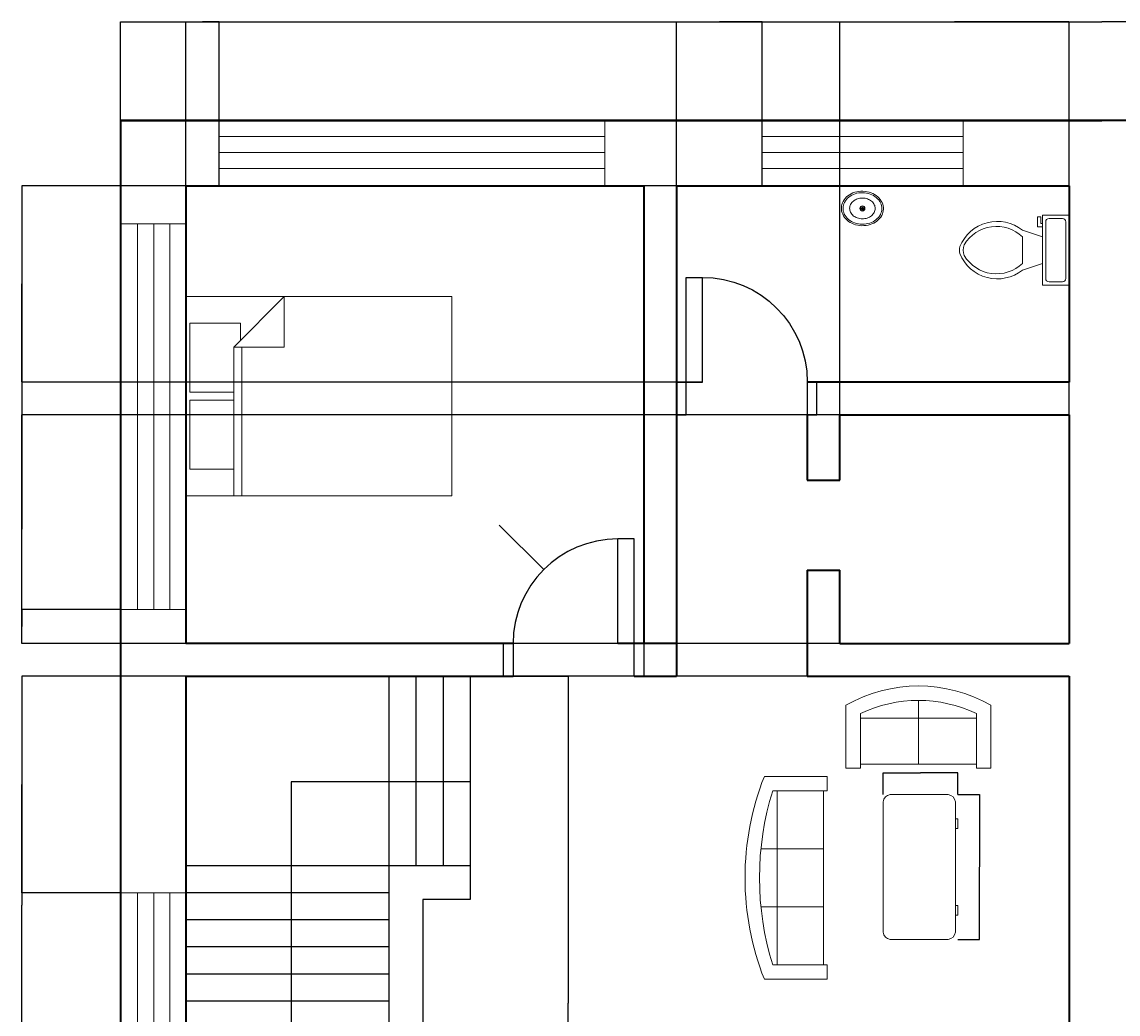
# Model space of a CAD drawing. Units: millimetres. Extents: x 726 to 37095, y -1634 to 13537.
# Tile 3 of 4: x 20550 to 28928, y 5952 to 13537. Entities that reach past the tile are written whole.
import ezdxf

# ---------------------------------------------------------------- set-up
doc = ezdxf.new("R2010")
doc.units = ezdxf.units.MM
for name, color, linetype, lineweight in [('A-ANNO-DIMS', 2, 'Continuous', 18), ('A-DOOR', 3, 'Continuous', 25), ('A-FLOR-FIXT', 9, 'Continuous', 18), ('A-FLOR-STRS', 5, 'Continuous', 25), ('A-FURN', 8, 'Continuous', 18), ('A-GLAZ', 4, 'Continuous', 18), ('A-WALL', 7, 'Continuous', 35)]:
    doc.layers.add(name, color=color, linetype=linetype, lineweight=lineweight)
doc.styles.get("Standard").update_dxf_attribs({"font": 'arial.ttf'})
doc.dimstyles.get("Standard").update_dxf_attribs({"dimtxt": 0.18, "dimasz": 0.18, "dimexe": 0.18, "dimexo": 0.0625, "dimgap": 0.09, "dimtad": 0, "dimtih": 1, "dimtoh": 1, "dimdec": 4, "dimzin": 0, "dimdsep": 46, "dimtxsty": 'Standard', "dimcen": 0.09, "dimadec": 0, "dimazin": 0, "dimtfac": 1, "dimtdec": 4, "dimtofl": 0, "dimtmove": 0, "dimatfit": 3, "dimfxl": 1, "dimtolj": 1, "dimtzin": 0, "dimarcsym": 0})

# ---------------------------------------------------------------- blocks, each defined once
blk = doc.blocks.new('Bed - Queen')
for p, q in [((0, -80.00003000000002), (0, 0)), ((0, 0), (59.99998999999999, 0)), ((59.99998999999999, 0), (59.99998999999999, -80.00003000000002)), ((7.99999, -1.200000000000017), (28.79998, -1.200000000000017)), ((7.99999, -14.4), (7.99999, -1.200000000000017)), ((28.79998, -1.200000000000017), (28.79998, -14.4)), ((31.19999, -1.200000000000017), (51.99999000000001, -1.200000000000017)), ((31.19999, -14.4), (31.19999, -1.200000000000017)), ((51.99999000000001, -1.200000000000017), (51.99999000000001, -16.4)), ((0, -14.4), (44.79999999999999, -14.4)), ((59.99998999999999, -29.60000000000001), (44.79999999999999, -14.4)), ((44.79999999999999, -14.4), (44.79999999999999, -29.60000000000001)), ((51.99999000000001, -16.4), (46.79936, -16.4)), ((44.79999999999999, -16.80000000000001), (0, -16.80000000000001)), ((44.79999999999999, -29.60000000000001), (59.99998999999999, -29.60000000000001)), ((59.99998999999999, -80.00003000000002), (0, -80.00003000000002))]:
    blk.add_line(p, q)
blk = doc.blocks.new('Window - Wood Frame 36 in. Wide plan')
for p, q in [((0, 6), (0, 0)), ((36, 6), (36, 0)), ((0, 4.5), (36, 4.5)), ((0, 3), (36, 3)), ((0, 1.5), (36, 1.5))]:
    blk.add_line(p, q)
blk = doc.blocks.new('Sofa - Roundback 7 ft.')
for p, q in [((-12.00002, -32.44210000000393), (-12.00003, -6.597100000003898)), ((11.99996999999999, -32.44210000000393), (11.99997999999999, -6.597100000003898)), ((-36.000027, -34.00000000000395), (-36.000027, -11.46960000000396)), ((-35.999844, -13.38190000000397), (35.99979999999999, -13.38190000000397)), ((35.99997999999999, -34.00000000000395), (35.99997999999999, -11.46960000000396)), ((-36.000027, -32.44210000000393), (35.99997999999999, -32.44210000000393))]:
    blk.add_line(p, q)
for points in [[(-36.000027, -34.00000000000395), (-42.000027, -34.00000000000395), (-42.000027, -8.000000000003944)], [(41.99997999999999, -8.000000000003944), (41.99997999999999, -34.00000000000395), (35.99997999999999, -34.00000000000395)]]:
    blk.add_lwpolyline(points)
for centre, radius, start, end in [((0, -114.2500000000039), 114.2500000000039, 68.43141000000072, 111.5686000000006), ((-1.00000000032e-05, -127.1968000000039), 121.1967999999973, 72.72032999999948, 107.2797000000005)]:
    blk.add_arc(centre, radius, start, end)
blk = doc.blocks.new('Desk - 30 x 60 in.')
for p, q in [((-26.999995, 0), (26.999995, 0)), ((-29.999995, -27), (-29.999995, -3)), ((29.999995, -3), (29.999995, -27)), ((26.999995, -30), (-26.999995, -30)), ((-20.000005, -30), (-20.000005, -31)), ((-20.000005, -31), (-16.000005, -31)), ((-16.000005, -31), (-16.000005, -30)), ((15.999995, -31), (15.999995, -30)), ((19.999995, -31), (15.999995, -31)), ((19.999995, -30), (19.999995, -31))]:
    blk.add_line(p, q)
for centre, radius, start, end in [((-26.499995, -3.5), 3.535534000004229, 98.1300999999916, 171.8698999999352), ((26.499995, -3.5), 3.535533999997753, 8.130102000022115, 81.8698999999439), ((-26.499995, -26.5), 3.535534000000845, 188.1301000000653, 261.8699000000085), ((26.499995, -26.5), 3.535534000004826, 278.1301000000561, 351.8698999999439)]:
    blk.add_arc(centre, radius, start, end)
blk = doc.blocks.new('Sofa - Roundback Loveseat 5 ft.')
for p, q in [((0, -32.44198000000246), (0, -5.999980000002448)), ((-23.99999999999999, -33.99998000000245), (-23.99999999999999, -11.46958000000243)), ((-23.99979999999998, -13.38178000000245), (23.99986, -13.38178000000245)), ((24.00004000000001, -33.99998000000245), (24.00004000000001, -11.46958000000243)), ((-23.99999999999999, -32.44198000000246), (24.00004000000001, -32.44198000000246))]:
    blk.add_line(p, q)
for points in [[(-23.99999999999999, -33.99998000000245), (-29.99999999999999, -33.99998000000245), (-29.99999999999999, -7.999980000002448)], [(30.00004000000001, -7.999980000002448), (30.00004000000001, -33.99998000000245), (24.00004000000001, -33.99998000000245)]]:
    blk.add_lwpolyline(points)
for centre, radius, start, end in [((0, -60.24998000000245), 60.24998000000245, 60.13715000000122, 119.862800000004), ((0, -61.38438000000245), 55.38444000000723, 64.32083000000306, 115.6791999999996)]:
    blk.add_arc(centre, radius, start, end)
blk = doc.blocks.new('Toilet - top')
for p, q in [((9.5, -6), (9.5, -2)), ((-10, -8.5), (-8, -8.5)), ((-10, -9.5), (-10, -8.5)), ((-7, -9.5), (-10, -9.5)), ((-8, -8.5), (-8, -8)), ((-7, -8), (-7, -9.5)), ((-4, -8), (-6, -14)), ((4, -8), (6, -14)), ((4, -14), (-4, -14))]:
    blk.add_line(p, q)
blk.add_lwpolyline([(10.5, -8), (10.5, 0), (-10.5, 0), (-10.5, -8)], close=True)
for points in [[(-9.5, -2), (-9.5, -6)], [(8.5, -1), (-8.5, -1)], [(-8.5, -7), (8.5, -7)]]:
    blk.add_lwpolyline(points)
for centre, radius, start, end in [((-8.625, -1.875), 0.8838834999999999, 81.86989999999999, 188.1301), ((8.625, -1.875), 0.8838834999999999, 351.8699, 98.13009999999998), ((-8.625, -6.125), 0.8838834999999999, 171.869898, 278.1301), ((8.625, -6.125), 0.8838834999999999, 261.8699, 8.130099999999993), ((3.519562435188956, -21.58049502388982), 12.16902005083646, 141.4691096810948, 247.9714346835576), ((4.199957580658807, -21.81740929088453), 11.3291791325804, 136.3677254423718, 238.946823937405), ((-3.519499936778316, -21.58047137067522), 12.16903423757823, 292.0284332733152, 38.53070636800453), ((-4.199890672038477, -21.81738596564128), 11.32918622148567, 301.0530065773863, 43.63209216694732), ((2.09660981727e-05, -27.87646475467881), 4, 245.7318247449371, 294.2681740488959), ((2.09415214183e-05, -28.99996806116075), 4, 254.8605283244437, 285.1394707718433)]:
    blk.add_arc(centre, radius, start, end)
blk = doc.blocks.new('Sink - Oval top')
for p, q in [((-1, 0), (1, 0)), ((0, 1), (0, -1))]:
    blk.add_line(p, q)
for points in [[(-12.23371880354079, 0.3941914712607968, 0.1176342565883263), (-11.46456229543957, -3.361933235489118, 0.104469279667093), (-8.878748691070427, -6.803541973650567, 0.0900157896014849), (-5.082757700676665, -9.072309807490512, 0.0819199491592185), (-0.3227280122732736, -10.01585280257211, 0.0819199491592091), (4.488169920880977, -9.380701564817912, 0.0900157896014801), (8.422342359155778, -7.36101289847943, 0.1044692796670922), (11.22435122606941, -4.093009071543406, 0.1176342565883338), (12.23371880354091, -0.3941914712607968, 0.1176342565883057), (11.46456229543992, 3.361933235488777, 0.1044692796670849), (8.878748691070427, 6.803541973650567, 0.0900157896014884), (5.082757700676324, 9.072309807490681, 0.0819199491592058), (0.3227280122732736, 10.01585280257211, 0.081919949159207), (-4.488169920880864, 9.380701564817969, 0.0900157896014802), (-8.422342359155778, 7.36101289847943, 0.1044692796670951), (-11.22435122606919, 4.093009071543633, 0.1176342565883402)], [(-11.28627986850119, 0.1590597164737346, 0.1186217001864142), (-10.51590095791209, -3.253161772358112, 0.1046781721811095), (-8.071803350560115, -6.358618019863342, 0.0895620664691738), (-4.537699193222351, -8.366971929609804, 0.0811846988912177), (-0.1289739026695997, -9.15150355811437, 0.0811846988912276), (4.300109150126218, -8.491524865184601, 0.0895620664691798), (7.889406708212618, -6.583562428127606, 0.1046781721811044), (10.42004782883111, -3.548216131892445, 0.1186217001864013), (11.28627986850119, -0.1590597164736209, 0.1186217001863945), (10.51590095791221, 3.253161772357998, 0.1046781721811069), (8.071803350560115, 6.358618019863342, 0.0895620664691756), (4.537699193222124, 8.366971929609917, 0.081184698891216), (0.1289739026695997, 9.151503558114428, 0.0811846988912142), (-4.300109150125877, 8.491524865184829, 0.0895620664691747), (-7.889406708212618, 6.583562428127606, 0.1046781721811045), (-10.42004782883111, 3.548216131892445, 0.1186217001863946)], [(-7.420452389032902, 0.0829876781601797, 0.1182825673856775), (-6.907065465214486, -2.1674649380775, 0.1046074595377274), (-5.294791470712084, -4.209988192029413, 0.0897179636260996), (-2.966599981142508, -5.528122152688069, 0.0814360825277113), (-0.0675135187855176, -6.036810076758797, 0.0814360825277218), (2.84222437824053, -5.593085960977873, 0.0897179636261315), (5.199312936802016, -4.327350491993342, 0.1046074595376878), (6.85686365682659, -2.321395784920355, 0.1182825673856714), (7.420452389033016, -0.0829876781601797, 0.1182825673856961), (6.907065465214486, 2.167464938077614, 0.1046074595377135), (5.294791470712084, 4.209988192029413, 0.0897179636261265), (2.966599981142621, 5.528122152687842, 0.0814360825277426), (0.0675135187855176, 6.036810076758797, 0.0814360825277225), (-2.842224378240644, 5.593085960977873, 0.0897179636261212), (-5.199312936802016, 4.327350491993342, 0.1046074595377049), (-6.856863656826476, 2.321395784920355, 0.1182825673856712)]]:
    blk.add_lwpolyline(points, format="xyb", close=True)
for radius in [1.5, 1]:
    blk.add_circle((0, 0), radius)
blk = doc.blocks.new('DOOR-SWING-800')
for p, q in [((999.1999999999979, 1050), (874.1999999999979, 1050)), ((874.1999999999979, 250), (874.1999999999979, 1050)), ((999.1999999999979, 250), (999.1999999999979, 1050)), ((9.095e-13, 250), (74.199999999998, 250)), ((9.095e-13, 0), (9.095e-13, 250)), ((74.199999999998, 250), (74.199999999998, 0)), ((874.1999999999979, 250), (999.1999999999979, 250)), ((999.1999999999979, 250), (1073.400000000002, 250)), ((999.1999999999979, 0), (999.1999999999979, 250)), ((1073.400000000002, 250), (1073.400000000002, 0)), ((74.199999999998, 0), (9.095e-13, 0)), ((1073.400000000002, 0), (999.1999999999979, 0))]:
    blk.add_line(p, q)
blk.add_arc((874.1999999999979, 250), 800, 90, 180)
blk = doc.blocks.new('STAIR-QUARTER-TURN')
for p, q in [((1551.94660387568, 5000.000000000002), (1551.94660387568, 3551.516503049365)), ((1758.872817725773, 5000.000000000002), (1758.872817725773, 3551.516503049365)), ((1965.799031575862, 5000.000000000002), (1965.799031575862, 3551.516503049365)), ((2172.725245425954, 5000.000000000002), (2172.725245425954, 3551.516503049365)), ((2172.725245425954, 4193.579423830473), (803.743340616409, 4193.579423830471)), ((803.743340616409, 4193.579423830471), (803.743340616409, 330.5564002077117)), ((2172.725245425954, 3551.516503049366), (0, 3551.516503049365)), ((1551.94660387568, 3551.516503049365), (1551.94660387568, 3344.590289199272)), ((2172.725245425954, 3551.516503049365), (2172.725245425954, 3292.858735736751)), ((1551.94660387568, 3344.590289199272), (0, 3344.590289199273)), ((1551.94660387568, 3344.590289199272), (1551.94660387568, 861.4757229981805)), ((2172.725245425954, 3292.858735736751), (1810.604371188295, 3292.858735736751)), ((1810.604371188295, 3292.85873573675), (1810.604371188295, 602.8179556856148)), ((1551.94660387568, 3137.664075349182), (0, 3137.664075349182)), ((1551.94660387568, 2930.73786149909), (0, 2930.737861499091)), ((1551.94660387568, 2723.811647649), (0, 2723.811647649001)), ((1551.94660387568, 2516.885433798908), (0, 2516.885433798909)), ((1551.94660387568, 2309.959219948817), (0, 2309.959219948818)), ((1551.94660387568, 2103.033006098726), (0, 2103.033006098727)), ((1551.94660387568, 1896.106792248635), (0, 1896.106792248635)), ((1551.94660387568, 1689.180578398543), (0, 1689.180578398544)), ((1551.94660387568, 1482.254364548453), (0, 1482.254364548454)), ((1551.94660387568, 1275.328150698362), (0, 1275.328150698363)), ((1551.94660387568, 1068.40193684827), (0, 1068.401936848271)), ((1551.94660387568, 861.4757229981795), (0, 861.4757229981805)), ((1551.94660387568, 861.4757229981805), (1551.946603875687, 602.8179556856074)), ((1810.604371188295, 602.8179556856148), (1551.946603875687, 602.8179556855675)), ((803.743340616409, 330.5564002077117), (545.0855733037969, 330.5564002077117)), ((545.0855733037969, 330.5564002077117), (803.743340616409, 4.547e-13)), ((803.743340616409, 330.5564002077117), (1062.401107929021, 330.5564002077108)), ((803.743340616409, 4.547e-13), (1062.401107929021, 330.5564002077117))]:
    blk.add_line(p, q)
blk = doc.blocks.new('WIN-1535')
for p, q in [((0, 1.819e-12), (0, 500.0000000000036)), ((1534.861597237876, 1.819e-12), (1534.861597237876, 500.0000000000036)), ((-9.095e-13, 377.1532172399693), (1534.861597237876, 377.1532172399693)), ((-9.095e-13, 254.306434479935), (1534.861597237876, 254.306434479935)), ((-9.095e-13, 131.459651719897), (1534.861597237876, 131.4596517198988))]:
    blk.add_line(p, q)
blk = doc.blocks.new('*D29')
at = {"layer": 'A-ANNO-DIMS', "color": 0, "lineweight": -2, "transparency": 16777216}
for p, q in [((27704.03518192463, 7629.827471204357), (27870.29711232547, 7629.827471204357)), ((27870.11711232547, 7629.647471204356), (27870.11711232547, 7076.195772778692)), ((27870.11711232547, 6522.377935198867), (27870.11711232547, 7075.829633624531)), ((27704.03518192463, 6522.197935198867), (27870.29711232547, 6522.197935198867))]:
    blk.add_line(p, q, dxfattribs=at)
at = {"layer": 'A-ANNO-DIMS', "color": 0, "transparency": 16777216}
for points in [[(27870.08711232547, 7629.647471204356), (27870.14711232546, 7629.647471204356), (27870.11711232547, 7629.827471204357)], [(27870.08711232547, 6522.377935198867), (27870.14711232546, 6522.377935198867), (27870.11711232547, 6522.197935198867)]]:
    blk.add_solid(points, dxfattribs=at)
at = {"layer": 'Defpoints', "color": 0, "transparency": 16777216}
for p in [(27703.97268192463, 7629.827471204357), (27870.11711232547, 7629.827471204357), (27703.97268192463, 6522.197935198867)]:
    blk.add_point(p, dxfattribs=at)
at = {"layer": 'A-ANNO-DIMS', "color": 0, "transparency": 16777216, "insert": (27870.11711232546, 7076.012703201602), "char_height": 0.18, "attachment_point": 5}
blk.add_mtext('\\A1;DESK 1108 TYP.', dxfattribs=at)
blk = doc.blocks.new('*D30')
at = {"layer": 'A-ANNO-DIMS', "color": 0, "lineweight": -2, "transparency": 16777216}
for p, q in [((27131.69732634582, 7629.889971204353), (27131.69732634582, 7796.151901605177)), ((27131.87732634582, 7795.971901605176), (27417.2369891284, 7795.971901605176)), ((27703.79268192461, 7795.971901605176), (27418.43301914204, 7795.971901605176)), ((27703.97268192462, 7629.889971204353), (27703.97268192462, 7796.151901605177))]:
    blk.add_line(p, q, dxfattribs=at)
at = {"layer": 'A-ANNO-DIMS', "color": 0, "transparency": 16777216}
for points in [[(27131.87732634582, 7796.001901605176), (27131.87732634582, 7795.941901605177), (27131.69732634582, 7795.971901605176)], [(27703.79268192461, 7796.001901605176), (27703.79268192461, 7795.941901605177), (27703.97268192462, 7795.971901605176)]]:
    blk.add_solid(points, dxfattribs=at)
at = {"layer": 'Defpoints', "color": 0, "transparency": 16777216}
for p in [(27131.69732634582, 7795.971901605176), (27131.69732634582, 7629.827471204354), (27703.97268192462, 7629.827471204354)]:
    blk.add_point(p, dxfattribs=at)
at = {"layer": 'A-ANNO-DIMS', "color": 0, "transparency": 16777216, "insert": (27417.83500413522, 7795.971901605176), "char_height": 0.18, "attachment_point": 5}
blk.add_mtext('\\A1;572 TYP.', dxfattribs=at)
blk = doc.blocks.new('*D35')
at = {"layer": 'A-ANNO-DIMS', "color": 0, "lineweight": -2, "transparency": 16777216}
for p, q in [((23976.18779894455, 8533.885868122888), (24726.30529894457, 8533.885868122888)), ((24726.12529894457, 8533.705868122888), (24726.12529894457, 6034.068937699966)), ((24726.12529894457, 3534.065868122886), (24726.12529894457, 6033.702798545806)), ((23976.18779894455, 3533.885868122886), (24726.30529894458, 3533.885868122886))]:
    blk.add_line(p, q, dxfattribs=at)
at = {"layer": 'A-ANNO-DIMS', "color": 0, "transparency": 16777216}
for points in [[(24726.09529894457, 8533.705868122888), (24726.15529894457, 8533.705868122888), (24726.12529894457, 8533.885868122888)], [(24726.09529894458, 3534.065868122886), (24726.15529894457, 3534.065868122886), (24726.12529894457, 3533.885868122886)]]:
    blk.add_solid(points, dxfattribs=at)
at = {"layer": 'Defpoints', "color": 0, "transparency": 16777216}
for p in [(23976.12529894455, 8533.885868122888), (24726.12529894457, 8533.885868122888), (23976.12529894455, 3533.885868122886)]:
    blk.add_point(p, dxfattribs=at)
at = {"layer": 'A-ANNO-DIMS', "color": 0, "transparency": 16777216, "insert": (24726.12529894457, 6033.885868122878), "char_height": 0.18, "attachment_point": 5}
blk.add_mtext('\\A1;STAIR 5000 TYP.', dxfattribs=at)
blk = doc.blocks.new('*D63')
at = {"layer": 'A-ANNO-DIMS', "color": 0, "lineweight": -2, "transparency": 16777216}
for p, q in [((21303.400054, 12783.948368), (21303.400054, 13536.815868)), ((21303.580054, 13536.635868), (28802.98013585539, 13536.635868)), ((36303.220054, 13536.635868), (28803.81997214461, 13536.635868)), ((36303.400054, 12783.948368), (36303.400054, 13536.815868))]:
    blk.add_line(p, q, dxfattribs=at)
at = {"layer": 'A-ANNO-DIMS', "color": 0, "transparency": 16777216}
for points in [[(21303.580054, 13536.665868), (21303.580054, 13536.605868), (21303.400054, 13536.635868)], [(36303.220054, 13536.665868), (36303.220054, 13536.605868), (36303.400054, 13536.635868)]]:
    blk.add_solid(points, dxfattribs=at)
at = {"layer": 'Defpoints', "color": 0, "transparency": 16777216}
for p in [(36303.400054, 13536.635868), (21303.400054, 12783.885868), (36303.400054, 12783.885868)]:
    blk.add_point(p, dxfattribs=at)
at = {"layer": 'A-ANNO-DIMS', "color": 0, "transparency": 16777216, "insert": (28803.400054, 13536.635868), "char_height": 0.18, "attachment_point": 5}
blk.add_mtext('\\A1;15000', dxfattribs=at)
blk = doc.blocks.new('*D69')
at = {"layer": 'A-ANNO-DIMS', "color": 0, "lineweight": -2, "transparency": 16777216}
for p, q in [((25303.33755400002, 12283.885868), (20550.47005400002, 12283.885868)), ((20550.65005400002, 12283.705868), (20550.65005400002, 10534.06783252933)), ((20550.65005400002, 8784.065868000003), (20550.65005400002, 10533.70390347067)), ((25303.33755400002, 8783.885868000005), (20550.47005400002, 8783.885868000005))]:
    blk.add_line(p, q, dxfattribs=at)
at = {"layer": 'A-ANNO-DIMS', "color": 0, "transparency": 16777216}
for points in [[(20550.62005400002, 12283.705868), (20550.68005400002, 12283.705868), (20550.65005400002, 12283.885868)], [(20550.62005400002, 8784.065868000003), (20550.68005400002, 8784.065868000003), (20550.65005400002, 8783.885868000005)]]:
    blk.add_solid(points, dxfattribs=at)
at = {"layer": 'Defpoints', "color": 0, "transparency": 16777216}
for p in [(20550.65005400002, 12283.885868), (25303.40005400002, 12283.885868), (25303.40005400002, 8783.885868000005)]:
    blk.add_point(p, dxfattribs=at)
at = {"layer": 'A-ANNO-DIMS', "color": 0, "transparency": 16777216, "insert": (20550.65005400002, 10533.88586799999), "char_height": 0.18, "attachment_point": 5}
blk.add_mtext('\\A1;3500', dxfattribs=at)
blk = doc.blocks.new('*D70')
at = {"layer": 'A-ANNO-DIMS', "color": 0, "lineweight": -2, "transparency": 16777216}
for p, q in [((25553.33755400002, 12283.885868), (20550.47005400002, 12283.885868)), ((20550.65005400002, 12283.705868), (20550.65005400002, 11534.06777113779)), ((20550.65005400002, 10784.065868), (20550.65005400002, 11533.70396486221)), ((25553.33755400002, 10783.885868), (20550.47005400002, 10783.885868))]:
    blk.add_line(p, q, dxfattribs=at)
at = {"layer": 'A-ANNO-DIMS', "color": 0, "transparency": 16777216}
for points in [[(20550.62005400002, 12283.705868), (20550.68005400002, 12283.705868), (20550.65005400002, 12283.885868)], [(20550.62005400002, 10784.065868), (20550.68005400002, 10784.065868), (20550.65005400002, 10783.885868)]]:
    blk.add_solid(points, dxfattribs=at)
at = {"layer": 'Defpoints', "color": 0, "transparency": 16777216}
for p in [(25553.40005400002, 12283.885868), (20550.65005400002, 10783.885868), (25553.40005400002, 10783.885868)]:
    blk.add_point(p, dxfattribs=at)
at = {"layer": 'A-ANNO-DIMS', "color": 0, "transparency": 16777216, "insert": (20550.65005400002, 11533.88586799999), "char_height": 0.18, "attachment_point": 5}
blk.add_mtext('\\A1;1500', dxfattribs=at)
blk = doc.blocks.new('*D71')
at = {"layer": 'A-ANNO-DIMS', "color": 0, "lineweight": -2, "transparency": 16777216}
for p, q in [((26802.600054, 10533.948368), (26802.600054, 13536.815868)), ((26802.780054, 13536.635868), (27677.54471293588, 13536.635868)), ((28553.220054, 13536.635868), (27678.45539506412, 13536.635868)), ((28553.400054, 10533.948368), (28553.400054, 13536.815868))]:
    blk.add_line(p, q, dxfattribs=at)
at = {"layer": 'A-ANNO-DIMS', "color": 0, "transparency": 16777216}
for points in [[(26802.780054, 13536.665868), (26802.780054, 13536.605868), (26802.600054, 13536.635868)], [(28553.220054, 13536.665868), (28553.220054, 13536.605868), (28553.400054, 13536.635868)]]:
    blk.add_solid(points, dxfattribs=at)
at = {"layer": 'Defpoints', "color": 0, "transparency": 16777216}
for p in [(28553.400054, 13536.635868), (26802.600054, 10533.885868), (28553.400054, 10533.885868)]:
    blk.add_point(p, dxfattribs=at)
at = {"layer": 'A-ANNO-DIMS', "color": 0, "transparency": 16777216, "insert": (27678.000054, 13536.635868), "char_height": 0.18, "attachment_point": 5}
blk.add_mtext('\\A1;1750.8', dxfattribs=at)
blk = doc.blocks.new('*D72')
at = {"layer": 'A-ANNO-DIMS', "color": 0, "lineweight": -2, "transparency": 16777216}
for p, q in [((28553.33755400002, 10533.885868), (20550.47005400002, 10533.885868)), ((20550.65005400002, 10533.705868), (20550.65005400002, 9659.067771137792)), ((20550.65005400002, 8784.065868000003), (20550.65005400002, 9658.703964862214)), ((28553.33755400002, 8783.885868000005), (20550.47005400002, 8783.885868000005))]:
    blk.add_line(p, q, dxfattribs=at)
at = {"layer": 'A-ANNO-DIMS', "color": 0, "transparency": 16777216}
for points in [[(20550.62005400002, 10533.705868), (20550.68005400002, 10533.705868), (20550.65005400002, 10533.885868)], [(20550.62005400002, 8784.065868000003), (20550.68005400002, 8784.065868000003), (20550.65005400002, 8783.885868000005)]]:
    blk.add_solid(points, dxfattribs=at)
at = {"layer": 'Defpoints', "color": 0, "transparency": 16777216}
for p in [(28553.40005400002, 10533.885868), (20550.65005400002, 8783.885868000005), (28553.40005400002, 8783.885868000005)]:
    blk.add_point(p, dxfattribs=at)
at = {"layer": 'A-ANNO-DIMS', "color": 0, "transparency": 16777216, "insert": (20550.65005400002, 9658.885867999996), "char_height": 0.18, "attachment_point": 5}
blk.add_mtext('\\A1;1750', dxfattribs=at)
blk = doc.blocks.new('*D73')
at = {"layer": 'A-ANNO-DIMS', "color": 0, "lineweight": -2, "transparency": 16777216}
for p, q in [((28553.33755400002, 8533.885868000005), (20550.47005400001, 8533.885868000005)), ((20550.65005400001, 8533.705868000003), (20550.65005400002, 6784.067832529334)), ((20550.65005400002, 5034.065868000002), (20550.65005400002, 6783.70390347067)), ((28553.33755400002, 5033.885868000002), (20550.47005400002, 5033.885868000002))]:
    blk.add_line(p, q, dxfattribs=at)
at = {"layer": 'A-ANNO-DIMS', "color": 0, "transparency": 16777216}
for points in [[(20550.62005400001, 8533.705868000003), (20550.68005400001, 8533.705868000003), (20550.65005400001, 8533.885868000005)], [(20550.62005400002, 5034.065868000002), (20550.68005400002, 5034.065868000002), (20550.65005400002, 5033.885868000002)]]:
    blk.add_solid(points, dxfattribs=at)
at = {"layer": 'Defpoints', "color": 0, "transparency": 16777216}
for p in [(20550.65005400001, 8533.885868000005), (28553.40005400002, 8533.885868000005), (28553.40005400002, 5033.885868000002)]:
    blk.add_point(p, dxfattribs=at)
at = {"layer": 'A-ANNO-DIMS', "color": 0, "transparency": 16777216, "insert": (20550.65005400001, 6783.885867999995), "char_height": 0.18, "attachment_point": 5}
blk.add_mtext('\\A1;3500', dxfattribs=at)
blk = doc.blocks.new('*D75')
at = {"layer": 'A-ANNO-DIMS', "color": 0, "lineweight": -2, "transparency": 16777216}
for p, q in [((28553.400054, 12283.948368), (28553.400054, 13536.815868)), ((28553.580054, 13536.635868), (28803.11151375444, 13536.635868)), ((29053.220054, 13536.635868), (28803.68859424557, 13536.635868)), ((29053.400054, 12283.948368), (29053.400054, 13536.815868))]:
    blk.add_line(p, q, dxfattribs=at)
at = {"layer": 'A-ANNO-DIMS', "color": 0, "transparency": 16777216}
for points in [[(28553.580054, 13536.665868), (28553.580054, 13536.605868), (28553.400054, 13536.635868)], [(29053.220054, 13536.665868), (29053.220054, 13536.605868), (29053.400054, 13536.635868)]]:
    blk.add_solid(points, dxfattribs=at)
at = {"layer": 'Defpoints', "color": 0, "transparency": 16777216}
for p in [(29053.400054, 13536.635868), (28553.400054, 12283.885868), (29053.400054, 12283.885868)]:
    blk.add_point(p, dxfattribs=at)
at = {"layer": 'A-ANNO-DIMS', "color": 0, "transparency": 16777216, "insert": (28803.400054, 13536.635868), "char_height": 0.18, "attachment_point": 5}
blk.add_mtext('\\A1;500', dxfattribs=at)
blk = doc.blocks.new('*D76')
at = {"layer": 'A-ANNO-DIMS', "color": 0, "lineweight": -2, "transparency": 16777216}
for p, q in [((25553.400054, 12283.948368), (25553.400054, 13536.815868)), ((25553.580054, 13536.635868), (25880.4339327367, 13536.635868)), ((26208.07657, 13536.635868), (25881.2226912633, 13536.635868)), ((26208.25657, 12283.948368), (26208.25657, 13536.815868))]:
    blk.add_line(p, q, dxfattribs=at)
at = {"layer": 'A-ANNO-DIMS', "color": 0, "transparency": 16777216}
for points in [[(25553.580054, 13536.665868), (25553.580054, 13536.605868), (25553.400054, 13536.635868)], [(26208.07657, 13536.665868), (26208.07657, 13536.605868), (26208.25657, 13536.635868)]]:
    blk.add_solid(points, dxfattribs=at)
at = {"layer": 'Defpoints', "color": 0, "transparency": 16777216}
for p in [(26208.25657, 13536.635868), (25553.400054, 12283.885868), (26208.25657, 12283.885868)]:
    blk.add_point(p, dxfattribs=at)
at = {"layer": 'A-ANNO-DIMS', "color": 0, "transparency": 16777216, "insert": (25880.828312, 13536.635868), "char_height": 0.18, "attachment_point": 5}
blk.add_mtext('\\A1;654.9', dxfattribs=at)
blk = doc.blocks.new('*D78')
at = {"layer": 'A-ANNO-DIMS', "color": 0, "lineweight": -2, "transparency": 16777216}
for p, q in [((21803.400054, 12283.948368), (21803.400054, 13536.815868)), ((21803.580054, 13536.635868), (21930.19670510437, 13536.635868)), ((22057.603097, 13536.635868), (21930.98644589564, 13536.635868)), ((22057.783097, 12292.561237), (22057.783097, 13536.815868))]:
    blk.add_line(p, q, dxfattribs=at)
at = {"layer": 'A-ANNO-DIMS', "color": 0, "transparency": 16777216}
for points in [[(21803.580054, 13536.665868), (21803.580054, 13536.605868), (21803.400054, 13536.635868)], [(22057.603097, 13536.665868), (22057.603097, 13536.605868), (22057.783097, 13536.635868)]]:
    blk.add_solid(points, dxfattribs=at)
at = {"layer": 'Defpoints', "color": 0, "transparency": 16777216}
for p in [(22057.783097, 13536.635868), (21803.400054, 12283.885868), (22057.783097, 12292.498737)]:
    blk.add_point(p, dxfattribs=at)
at = {"layer": 'A-ANNO-DIMS', "color": 0, "transparency": 16777216, "insert": (21930.5915755, 13536.635868), "char_height": 0.18, "attachment_point": 5}
blk.add_mtext('\\A1;254.4', dxfattribs=at)
blk = doc.blocks.new('*D80')
at = {"layer": 'A-ANNO-DIMS', "color": 0, "lineweight": -2, "transparency": 16777216}
for p, q in [((21803.33755400001, 8533.885868000005), (20550.47005400001, 8533.885868000005)), ((20550.65005400001, 8533.705868000003), (20550.65005400002, 7706.362915637793)), ((20550.65005400002, 6878.656157000005), (20550.65005400002, 7705.999109362213)), ((21311.95042200001, 6878.476157000005), (20550.47005400002, 6878.476157000005))]:
    blk.add_line(p, q, dxfattribs=at)
at = {"layer": 'A-ANNO-DIMS', "color": 0, "transparency": 16777216}
for points in [[(20550.62005400001, 8533.705868000003), (20550.68005400001, 8533.705868000003), (20550.65005400001, 8533.885868000005)], [(20550.62005400002, 6878.656157000005), (20550.68005400002, 6878.656157000005), (20550.65005400002, 6878.476157000005)]]:
    blk.add_solid(points, dxfattribs=at)
at = {"layer": 'Defpoints', "color": 0, "transparency": 16777216}
for p in [(20550.65005400001, 8533.885868000005), (21803.40005400001, 8533.885868000005), (21312.01292200001, 6878.476157000005)]:
    blk.add_point(p, dxfattribs=at)
at = {"layer": 'A-ANNO-DIMS', "color": 0, "transparency": 16777216, "insert": (20550.65005400001, 7706.181012499995), "char_height": 0.18, "attachment_point": 5}
blk.add_mtext('\\A1;1655.4', dxfattribs=at)
blk = doc.blocks.new('*D81')
at = {"layer": 'A-ANNO-DIMS', "color": 0, "lineweight": -2, "transparency": 16777216}
for p, q in [((21311.95042200001, 9045.622310000004), (20550.47005400002, 9045.622310000004)), ((20550.65005400002, 9045.442310000002), (20550.65005400002, 8914.935992137793)), ((20550.65005400002, 8784.065868000003), (20550.65005400002, 8914.572185862216)), ((21803.33755400001, 8783.885868000005), (20550.47005400002, 8783.885868000005))]:
    blk.add_line(p, q, dxfattribs=at)
at = {"layer": 'A-ANNO-DIMS', "color": 0, "transparency": 16777216}
for points in [[(20550.62005400002, 9045.442310000002), (20550.68005400002, 9045.442310000002), (20550.65005400002, 9045.622310000004)], [(20550.62005400002, 8784.065868000003), (20550.68005400002, 8784.065868000003), (20550.65005400002, 8783.885868000005)]]:
    blk.add_solid(points, dxfattribs=at)
at = {"layer": 'Defpoints', "color": 0, "transparency": 16777216}
for p in [(20550.65005400002, 9045.622310000004), (21312.01292200001, 9045.622310000004), (21803.40005400001, 8783.885868000005)]:
    blk.add_point(p, dxfattribs=at)
at = {"layer": 'A-ANNO-DIMS', "color": 0, "transparency": 16777216, "insert": (20550.65005400002, 8914.754088999995), "char_height": 0.18, "attachment_point": 5}
blk.add_mtext('\\A1;261.74', dxfattribs=at)
blk = doc.blocks.new('*D87')
at = {"layer": 'A-ANNO-DIMS', "color": 0, "lineweight": -2, "transparency": 16777216}
for p, q in [((24198.92343643046, 9688.982610369547), (24199.10343643046, 9688.982610369547)), ((24199.10343643046, 9688.982610369547), (24538.38738878816, 9349.69861122939)), ((25104.110054, 8783.885868000001), (25104.29005400001, 8783.885868000005)), ((25104.20005400001, 8783.795868000003), (25104.200054, 8783.975868000003))]:
    blk.add_line(p, q, dxfattribs=at)
at = {"layer": 'A-ANNO-DIMS', "color": 0, "transparency": 16777216}
blk.add_solid([(24538.40860199306, 9349.719824431362), (24538.36617558327, 9349.677398027416), (24538.51466800001, 9349.571332)], dxfattribs=at)
at = {"layer": 'Defpoints', "color": 0, "transparency": 16777216}
for p in [(24538.51466800001, 9349.571332), (25104.200054, 8783.885868000005)]:
    blk.add_point(p, dxfattribs=at)
at = {"layer": 'A-ANNO-DIMS', "color": 0, "transparency": 16777216, "insert": (24198.35488936361, 9688.982610369543), "char_height": 0.18, "attachment_point": 5}
blk.add_mtext('\\A1;6X R800', dxfattribs=at)

msp = doc.modelspace()

# ---------------------------------------------------------------- linework, layer by layer
at = {"layer": 'A-DOOR'}
for p, q in [((25553.40005351859, 10783.88586812288), (25553.40005351859, 10533.88586812288)), ((25553.40005351859, 10783.88586812288), (25752.60005351859, 10783.88586812288)), ((25553.40005351859, 10783.88586812288), (25553.40005351859, 10533.88586812288)), ((25752.60005351859, 10783.88586812288), (25553.40005351859, 10783.88586812288)), ((25627.6000535186, 10783.88586812288), (25752.60005351859, 10783.88586812288)), ((25553.40005351859, 10533.88586812288), (25627.6000535186, 10533.88586812288)), ((25553.4000535186, 10533.88586812288), (25627.6000535186, 10533.88586812288)), ((26552.6000535186, 10533.88586812288), (26626.80005351859, 10533.88586812288)), ((25229.20005351859, 8783.885868122885), (25104.20005351859, 8783.885868122885))]:
    msp.add_line(p, q, dxfattribs=at)
at = {"layer": 'A-WALL'}
for p, q in [((36303.40005351859, 12783.88586812288), (21303.40005351859, 12783.88586812288)), ((21303.40005351859, 12783.88586812288), (21303.40005351859, 2283.885868122887)), ((21303.40005351859, 12783.88586812288), (28803.40005351859, 12783.88586812288)), ((21803.40005351859, 12283.88586812288), (21803.40005351859, 8783.885868122885)), ((21803.40005351859, 12283.88586812288), (25303.40005351859, 12283.88586812288)), ((25303.40005351859, 12283.88586812288), (25303.40005351859, 8783.885868122885)), ((25553.40005351859, 12283.88586812288), (25553.40005351859, 9283.885868122885)), ((25553.40005351859, 12283.88586812288), (28553.40005351859, 12283.88586812288)), ((28553.40005351859, 12283.88586812288), (28553.40005351859, 10783.88586812288)), ((28553.4000535186, 10783.88586812288), (26552.6000535186, 10783.88586812288)), ((26552.6000535186, 10533.88586812288), (26552.6000535186, 10032.95383072874)), ((26802.6000535186, 10533.88586812288), (28553.40005351859, 10533.88586812288)), ((26802.6000535186, 10032.95383072874), (26802.6000535186, 10533.88586812288)), ((28553.40005351859, 10533.88586812288), (28553.40005351859, 8783.885868122883)), ((26552.6000535186, 10032.95383072874), (26802.6000535186, 10032.95383072874)), ((26552.6000535186, 9345.861970410639), (26802.6000535186, 9345.861970410639)), ((26552.6000535186, 9345.861970410639), (26552.6000535186, 8533.885868122887)), ((26802.6000535186, 8783.885868122883), (26802.6000535186, 9345.861970410639)), ((25553.40005351859, 9283.885868122885), (25553.40005351859, 9033.885868122885)), ((25553.40005351859, 9033.885868122885), (25553.40005351859, 8783.885868122885)), ((24304.20005351859, 8783.885868122885), (21803.40005351859, 8783.885868122885)), ((25303.40005351859, 8783.885868122885), (25104.20005351859, 8783.885868122885)), ((25553.40005351859, 8783.885868122885), (25303.40005351859, 8783.885868122885)), ((25553.40005351859, 8783.885868122885), (25553.40005351859, 8533.885868122887)), ((26802.6000535186, 8783.885868122883), (28553.40005351859, 8783.885868122885)), ((21803.40005351859, 8533.885868122883), (21803.40005351859, 2783.885868122886)), ((21803.40005351859, 8533.885868122885), (24304.20005351859, 8533.885868122885)), ((25229.20005351859, 8533.885868122887), (25553.4000535186, 8533.885868122887)), ((26552.6000535186, 8533.885868122888), (28553.40005351859, 8533.885868122885)), ((26552.6000535186, 8533.885868122887), (26802.6000535186, 8533.885868122887)), ((28553.40005351859, 8533.885868122887), (28553.40005351859, 5033.885868122885))]:
    msp.add_line(p, q, dxfattribs=at)

# ---------------------------------------------------------------- block references
at = {"layer": 'A-DOOR', "extrusion": (0, 0, -1), "zscale": -1}
msp.add_blockref('DOOR-SWING-800', (-26626.80005351859, 10533.88586812287), dxfattribs=at)
at = {"layer": 'A-DOOR'}
msp.add_blockref('DOOR-SWING-800', (24230.00005351859, 8533.885868122887), dxfattribs=at)
at = {"layer": 'A-FLOR-FIXT', "xscale": 13.14744327818227, "yscale": 13.14744327818227, "zscale": 13.14744327818227}
msp.add_blockref('Sink - Oval top', (26974.34049594012, 12110.79179875842), dxfattribs=at)
at = {"layer": 'A-FLOR-FIXT', "xscale": 25.4, "yscale": 25.4, "zscale": 25.4, "rotation": 270}
msp.add_blockref('Toilet - top', (28553.40005351859, 11792.07151678625), dxfattribs=at)
at = {"layer": 'A-FLOR-STRS'}
msp.add_blockref('STAIR-QUARTER-TURN', (21803.40005351859, 3533.885868122883), dxfattribs=at)
at = {"layer": 'A-FURN', "rotation": 90}
for name, p, xscale, yscale, zscale in [('Bed - Queen', (21803.40005351859, 9913.47188921653), 25.4, 25.4, 25.4), ('Sofa - Roundback 7 ft.', (26076.9867468829, 6993.391282043552), 18.46049527356076, 18.46049527356076, 18.46049527356076), ('Desk - 30 x 60 in.', (27131.69732844423, 7076.012703201602), 18.46049527356076, 18.46049527356076, 18.46049527356076)]:
    msp.add_blockref(name, p, dxfattribs=dict(at, xscale=xscale, yscale=yscale, zscale=zscale))
at = {"layer": 'A-FURN', "xscale": 18.46049527356076, "yscale": 18.46049527356076, "zscale": 18.46049527356076}
msp.add_blockref('Sofa - Roundback Loveseat 5 ft.', (27402.62229803196, 8460.12169162394), dxfattribs=at)
at = {"layer": 'A-GLAZ', "xscale": 81.8978551733564, "yscale": 81.8978551733564, "zscale": 81.8978551733564}
msp.add_blockref('Window - Wood Frame 36 in. Wide plan', (22057.7830971272, 12292.49873708274), dxfattribs=at)
at = {"layer": 'A-GLAZ'}
msp.add_blockref('WIN-1535', (26208.25656970763, 12283.88586812288), dxfattribs=at)
at = {"layer": 'A-GLAZ', "xscale": 81.8978551733564, "yscale": 81.8978551733564, "zscale": 81.8978551733564, "rotation": 270}
for p in [(21312.01292247845, 11993.94509580379), (21312.01292247845, 6878.476157322156)]:
    msp.add_blockref('Window - Wood Frame 36 in. Wide plan', p, dxfattribs=at)

# ---------------------------------------------------------------- dimensions: what is measured, and where the dimension line sits
at = {"layer": 'A-ANNO-DIMS'}
for base, p1, p2, override, picture, middle in [((36303.400054, 13536.635868), (21303.400054, 12783.885868), (36303.400054, 12783.885868), {"dimdec": 0, "dimlfac": 1, "dimrnd": 0, "dimzin": 0, "dimdsep": 46, "dimlunit": 2}, '*D63', (28803.400054, 13536.635868)), ((22057.783097, 13536.635868), (21803.400054, 12283.885868), (22057.783097, 12292.498737), {"dimdec": 1, "dimlfac": 1, "dimrnd": 0, "dimzin": 0, "dimdsep": 46, "dimlunit": 2}, '*D78', (21930.5915755, 13536.635868)), ((26208.25657, 13536.635868), (25553.400054, 12283.885868), (26208.25657, 12283.885868), {"dimdec": 1, "dimlfac": 1, "dimrnd": 0, "dimzin": 0, "dimdsep": 46, "dimlunit": 2}, '*D76', (25880.828312, 13536.635868)), ((28553.400054, 13536.635868), (26802.600054, 10533.885868), (28553.400054, 10533.885868), {"dimdec": 1, "dimlfac": 1, "dimrnd": 0, "dimzin": 0, "dimdsep": 46, "dimlunit": 2}, '*D71', (27678.000054, 13536.635868)), ((29053.400054, 13536.635868), (28553.400054, 12283.885868), (29053.400054, 12283.885868), {"dimdec": 0, "dimlfac": 1, "dimrnd": 0, "dimzin": 0, "dimdsep": 46, "dimlunit": 2}, '*D75', (28803.400054, 13536.635868))]:
    dim = msp.add_linear_dim(base=base, p1=p1, p2=p2, dimstyle='Standard', override=override, dxfattribs=at)
    dim.commit()
    dim.dimension.update_dxf_attribs({"geometry": picture, "text_midpoint": middle})
for base, p1, p2, override, picture, middle in [((20550.65005400002, 12283.885868), (25303.400054, 8783.885868), (25303.400054, 12283.885868), {"dimdec": 0, "dimlfac": 1, "dimrnd": 0, "dimzin": 0, "dimdsep": 46, "dimlunit": 2}, '*D69', (20550.65005400002, 10533.88586799999)), ((20550.65005400002, 10783.885868), (25553.400054, 12283.885868), (25553.400054, 10783.885868), {"dimdec": 0, "dimlfac": 1, "dimrnd": 0, "dimzin": 0, "dimdsep": 46, "dimlunit": 2}, '*D70', (20550.65005400002, 11533.88586799999)), ((20550.65005400002, 8783.885868000005), (28553.400054, 10533.885868), (28553.400054, 8783.885868), {"dimdec": 0, "dimlfac": 1, "dimrnd": 0, "dimzin": 0, "dimdsep": 46, "dimlunit": 2}, '*D72', (20550.65005400002, 9658.885867999996)), ((20550.65005400002, 9045.622310000004), (21803.400054, 8783.885868), (21312.012922, 9045.62231), {"dimdec": 2, "dimlfac": 1, "dimrnd": 0, "dimzin": 0, "dimdsep": 46, "dimlunit": 2}, '*D81', (20550.65005400002, 8914.754088999995)), ((20550.65005400001, 8533.885868000005), (21312.012922, 6878.476157), (21803.400054, 8533.885868), {"dimdec": 1, "dimlfac": 1, "dimrnd": 0, "dimzin": 0, "dimdsep": 46, "dimlunit": 2}, '*D80', (20550.65005400001, 7706.181012499995)), ((20550.65005400001, 8533.885868000005), (28553.400054, 5033.885868), (28553.400054, 8533.885868), {"dimdec": 0, "dimlfac": 1, "dimrnd": 0, "dimzin": 0, "dimdsep": 46, "dimlunit": 2}, '*D73', (20550.65005400001, 6783.885867999995))]:
    dim = msp.add_linear_dim(base=base, p1=p1, p2=p2, angle=90, dimstyle='Standard', override=override, dxfattribs=at)
    dim.commit()
    dim.dimension.update_dxf_attribs({"geometry": picture, "text_midpoint": middle})
dim = msp.add_radius_dim(center=(25104.200054, 8783.885868000005), mpoint=(24538.51466800001, 9349.571332), text='6X <>', dimstyle='Standard', override={"dimdec": 0, "dimlfac": 1, "dimrnd": 0, "dimzin": 0, "dimdsep": 46, "dimlunit": 2}, dxfattribs=at)
dim.commit()
dim.dimension.update_dxf_attribs({"geometry": '*D87', "text_midpoint": (24198.35488936361, 9688.982610369543), "dimtype": 164})
for base, p1, p2, angle, text, picture, middle in [((24726.12529894457, 8533.885868122888), (23976.12529894455, 3533.885868122883), (23976.12529894455, 8533.885868122885), 90, 'STAIR <> TYP.', '*D35', (24726.12529894457, 6033.885868122878)), ((27131.69732634582, 7795.971901605176), (27703.97268192462, 7629.827471204354), (27131.69732634582, 7629.827471204354), 180, '<> TYP.', '*D30', (27417.83500413522, 7795.971901605176)), ((27870.11711232547, 7629.827471204357), (27703.97268192462, 6522.197935198864), (27703.97268192462, 7629.827471204354), 90, 'DESK <> TYP.', '*D29', (27870.11711232546, 7076.012703201602))]:
    dim = msp.add_linear_dim(base=base, p1=p1, p2=p2, angle=angle, text=text, dimstyle='Standard', override={"dimdec": 0, "dimlfac": 1, "dimrnd": 0, "dimzin": 0, "dimdsep": 46, "dimlunit": 2}, dxfattribs=at)
    dim.commit()
    dim.dimension.update_dxf_attribs({"geometry": picture, "text_midpoint": middle})

doc.saveas('drawing.dxf')
